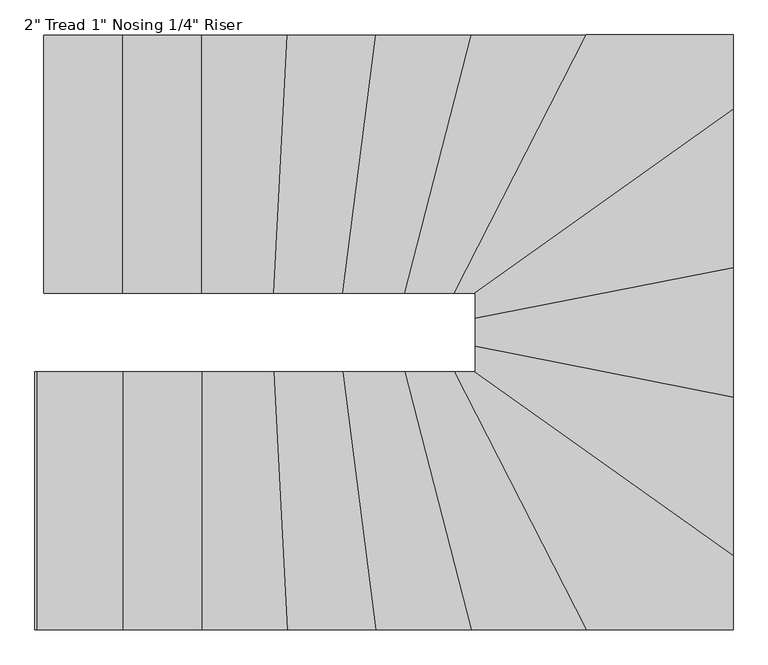
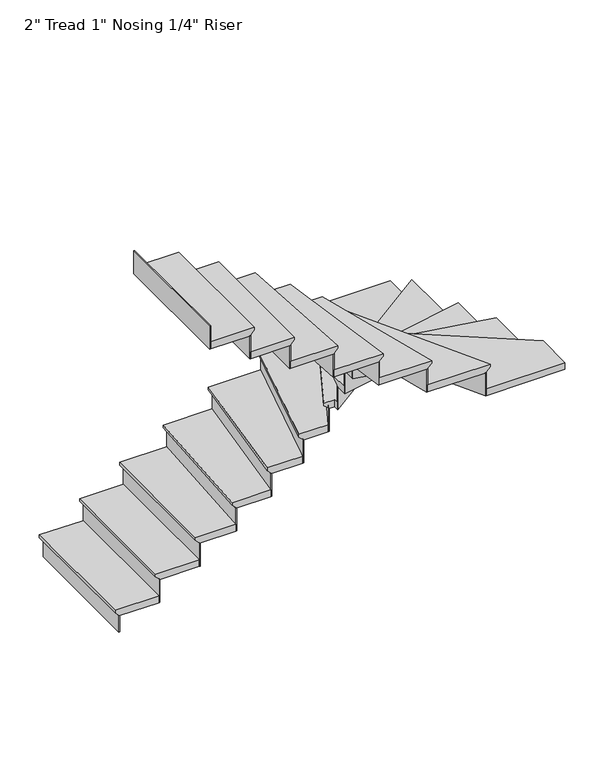
"""IFC4 building model written with IfcOpenShell, lengths in millimetres: stair flight geometry."""

from ifc_helpers import new_model, si_unit, origin, place, context, project, spatial, faceted_brep, source, transform, mapped, element, save


def stair_flight_813748e6(model_context):
    return source(origin(), model_context, "Body", "Brep", [
        faceted_brep([(-5314.5158104, 2778.8271763, 150.2833333), (-5314.5158104, 2778.8271763, 169.3333333), (-5314.5158104, 3693.2271763, 169.3333333), (-5314.5158104, 3693.2271763, 150.2833333), (-5289.1158104, 2778.8271763, 124.8833333), (-5289.1158104, 3693.2271763, 124.8833333), (-5009.7158104, 2778.8271763, 169.3333333), (-5009.7158104, 3693.2271763, 169.3333333), (-5289.1158104, 3693.2271763, 118.5333333), (-5009.7158104, 3693.2271763, 118.5333333), (-5009.7158104, 2778.8271763, 118.5333333), (-5289.1158104, 2778.8271763, 118.5333333)], [[[0, 1, 2, 3]], [[4, 0, 3, 5]], [[2, 1, 6, 7]], [[8, 9, 10, 11]], [[2, 7, 9, 8, 5, 3]], [[8, 11, 4, 5]], [[6, 1, 0, 4, 11, 10]], [[7, 6, 10, 9]]]),
        faceted_brep([(-5289.1158104, 2778.8271763, 118.5333333), (-5289.1158104, 2778.8271763, 0.0), (-5282.7658104, 2778.8271763, 0.0), (-5282.7658104, 2778.8271763, 118.5333333), (-5289.1158104, 3693.2271763, 118.5333333), (-5282.7658104, 3693.2271763, 118.5333333), (-5282.7658104, 3693.2271763, 0.0), (-5289.1158104, 3693.2271763, 0.0)], [[[0, 1, 2, 3]], [[4, 5, 6, 7]], [[1, 0, 4, 7]], [[2, 1, 7, 6]], [[3, 2, 6, 5]], [[0, 3, 5, 4]]]),
        faceted_brep([(-5009.7158104, 2778.8271763, 287.8666667), (-5009.7158104, 2778.8271763, 118.5333333), (-5003.3658104, 2778.8271763, 118.5333333), (-5003.3658104, 2778.8271763, 287.8666667), (-5009.7158104, 3693.2271763, 287.8666667), (-5003.3658104, 3693.2271763, 287.8666667), (-5003.3658104, 3693.2271763, 118.5333333), (-5009.7158104, 3693.2271763, 118.5333333)], [[[0, 1, 2, 3]], [[4, 5, 6, 7]], [[1, 0, 4, 7]], [[2, 1, 7, 6]], [[3, 2, 6, 5]], [[0, 3, 5, 4]]]),
        faceted_brep([(-5035.1158104, 3693.2271763, 338.6666667), (-5035.1158104, 2778.8271763, 338.6666667), (-4730.3158104, 2778.8271763, 338.6666667), (-4730.3158104, 3693.2271763, 338.6666667), (-5009.7158104, 3693.2271763, 287.8666667), (-4730.3158104, 3693.2271763, 287.8666667), (-4730.3158104, 2778.8271763, 287.8666667), (-5009.7158104, 2778.8271763, 287.8666667), (-5009.7158104, 3693.2271763, 294.2166667), (-5035.1158104, 3693.2271763, 319.6166667), (-5009.7158104, 2778.8271763, 294.2166667), (-5035.1158104, 2778.8271763, 319.6166667)], [[[0, 1, 2, 3]], [[4, 5, 6, 7]], [[0, 3, 5, 4, 8, 9]], [[4, 7, 10, 8]], [[2, 1, 11, 10, 7, 6]], [[3, 2, 6, 5]], [[11, 1, 0, 9]], [[10, 11, 9, 8]]]),
        faceted_brep([(-4730.3158104, 2778.8271763, 457.2), (-4730.3158104, 2778.8271763, 287.8666667), (-4723.9658104, 2778.8271763, 287.8666667), (-4723.9658104, 2778.8271763, 457.2), (-4730.3158104, 3693.2271763, 457.2), (-4723.9658104, 3693.2271763, 457.2), (-4723.9658104, 3693.2271763, 287.8666667), (-4730.3158104, 3693.2271763, 287.8666667)], [[[0, 1, 2, 3]], [[4, 5, 6, 7]], [[1, 0, 4, 7]], [[2, 1, 7, 6]], [[3, 2, 6, 5]], [[0, 3, 5, 4]]]),
        faceted_brep([(-4755.7158104, 3693.2271763, 508.0), (-4755.7158104, 2778.8271763, 508.0), (-4474.6486489, 2778.8271763, 508.0), (-4427.1143785, 3693.2271763, 508.0), (-4730.3158104, 3693.2271763, 457.2), (-4427.1143785, 3693.2271763, 457.2), (-4474.6486489, 2778.8271763, 457.2), (-4730.3158104, 2778.8271763, 457.2), (-4730.3158104, 3693.2271763, 463.55), (-4755.7158104, 3693.2271763, 488.95), (-4730.3158104, 2778.8271763, 463.55), (-4755.7158104, 2778.8271763, 488.95)], [[[0, 1, 2, 3]], [[4, 5, 6, 7]], [[0, 3, 5, 4, 8, 9]], [[4, 7, 10, 8]], [[2, 1, 11, 10, 7, 6]], [[3, 2, 6, 5]], [[11, 1, 0, 9]], [[10, 11, 9, 8]]]),
        faceted_brep([(-4474.6486489, 2778.8271763, 626.5333333), (-4474.6486489, 2778.8271763, 457.2), (-4468.2900747, 2778.8271763, 457.2), (-4468.2900747, 2778.8271763, 626.5333333), (-4427.1143785, 3693.2271763, 626.5333333), (-4420.7558043, 3693.2271763, 626.5333333), (-4420.7558043, 3693.2271763, 457.2), (-4427.1143785, 3693.2271763, 457.2)], [[[0, 1, 2, 3]], [[4, 5, 6, 7]], [[1, 0, 4, 7]], [[2, 1, 7, 6]], [[3, 2, 6, 5]], [[0, 3, 5, 4]]]),
        faceted_brep([(-4452.5486752, 3693.2271763, 677.3333333), (-4500.0829456, 2778.8271763, 677.3333333), (-4230.4819491, 2778.8271763, 677.3333333), (-4112.1258974, 3693.2271763, 677.3333333), (-4427.1143785, 3693.2271763, 626.5333333), (-4112.1258974, 3693.2271763, 626.5333333), (-4230.4819491, 2778.8271763, 626.5333333), (-4474.6486489, 2778.8271763, 626.5333333), (-4427.1143785, 3693.2271763, 632.8833333), (-4452.5486752, 3693.2271763, 658.2833333), (-4474.6486489, 2778.8271763, 632.8833333), (-4500.0829456, 2778.8271763, 658.2833333)], [[[0, 1, 2, 3]], [[4, 5, 6, 7]], [[0, 3, 5, 4, 8, 9]], [[4, 7, 10, 8]], [[2, 1, 11, 10, 7, 6]], [[3, 2, 6, 5]], [[11, 1, 0, 9]], [[10, 11, 9, 8]]]),
        faceted_brep([(-4230.4819491, 2778.8271763, 795.8666667), (-4230.4819491, 2778.8271763, 626.5333333), (-4224.0789773, 2778.8271763, 626.5333333), (-4224.0789773, 2778.8271763, 795.8666667), (-4112.1258974, 3693.2271763, 795.8666667), (-4105.7229256, 3693.2271763, 795.8666667), (-4105.7229256, 3693.2271763, 626.5333333), (-4112.1258974, 3693.2271763, 626.5333333)], [[[0, 1, 2, 3]], [[4, 5, 6, 7]], [[1, 0, 4, 7]], [[2, 1, 7, 6]], [[3, 2, 6, 5]], [[0, 3, 5, 4]]]),
        faceted_brep([(-4137.7377845, 3693.2271763, 846.6666667), (-4256.0938362, 2778.8271763, 846.6666667), (-4008.8547266, 2778.8271763, 846.6666667), (-3773.7242792, 3693.2271763, 846.6666667), (-4112.1258974, 3693.2271763, 795.8666667), (-3773.7242792, 3693.2271763, 795.8666667), (-4008.8547266, 2778.8271763, 795.8666667), (-4230.4819491, 2778.8271763, 795.8666667), (-4112.1258974, 3693.2271763, 802.2166667), (-4137.7377845, 3693.2271763, 827.6166667), (-4230.4819491, 2778.8271763, 802.2166667), (-4256.0938362, 2778.8271763, 827.6166667)], [[[0, 1, 2, 3]], [[4, 5, 6, 7]], [[0, 3, 5, 4, 8, 9]], [[4, 7, 10, 8]], [[2, 1, 11, 10, 7, 6]], [[3, 2, 6, 5]], [[11, 1, 0, 9]], [[10, 11, 9, 8]]]),
        faceted_brep([(-4008.8547266, 2778.8271763, 965.2), (-4008.8547266, 2778.8271763, 795.8666667), (-4002.2981497, 2778.8271763, 795.8666667), (-4002.2981497, 2778.8271763, 965.2), (-3773.7242792, 3693.2271763, 965.2), (-3767.1677023, 3693.2271763, 965.2), (-3767.1677023, 3693.2271763, 795.8666667), (-3773.7242792, 3693.2271763, 795.8666667)], [[[0, 1, 2, 3]], [[4, 5, 6, 7]], [[1, 0, 4, 7]], [[2, 1, 7, 6]], [[3, 2, 6, 5]], [[0, 3, 5, 4]]]),
        faceted_brep([(-3799.9505867, 3693.2271763, 1016.0), (-4035.0810341, 2778.8271763, 1016.0), (-3832.5080905, 2778.8271763, 1016.0), (-3363.6834692, 3693.2271763, 1016.0), (-3773.7242792, 3693.2271763, 965.2), (-3363.6834692, 3693.2271763, 965.2), (-3832.5080905, 2778.8271763, 965.2), (-4008.8547266, 2778.8271763, 965.2), (-3773.7242792, 3693.2271763, 971.55), (-3799.9505867, 3693.2271763, 996.95), (-4008.8547266, 2778.8271763, 971.55), (-4035.0810341, 2778.8271763, 996.95)], [[[0, 1, 2, 3]], [[4, 5, 6, 7]], [[0, 3, 5, 4, 8, 9]], [[4, 7, 10, 8]], [[2, 1, 11, 10, 7, 6]], [[3, 2, 6, 5]], [[11, 1, 0, 9]], [[10, 11, 9, 8]]]),
        faceted_brep([(-3832.5080905, 2778.8271763, 1134.5333333), (-3832.5080905, 2778.8271763, 965.2), (-3825.3721074, 2778.8271763, 965.2), (-3825.3721074, 2778.8271763, 1134.5333333), (-3363.6834692, 3693.2271763, 1134.5333333), (-3356.5474861, 3693.2271763, 1134.5333333), (-3356.5474861, 3693.2271763, 965.2), (-3363.6834692, 3693.2271763, 965.2)], [[[0, 1, 2, 3]], [[4, 5, 6, 7]], [[1, 0, 4, 7]], [[2, 1, 7, 6]], [[3, 2, 6, 5]], [[0, 3, 5, 4]]]),
        faceted_brep([(-2872.3841185, 3399.5460426, 1185.3333333), (-2872.3841185, 3693.2271763, 1185.3333333), (-3392.2274017, 3693.2271763, 1185.3333333), (-3861.0520231, 2778.8271763, 1185.3333333), (-3786.7841185, 2778.8271763, 1185.3333333), (-3786.7841185, 2749.2720934, 1185.3333333), (-2872.3841185, 3693.2271763, 1134.5333333), (-2872.3841185, 3399.5460426, 1134.5333333), (-3786.7841185, 2749.2720934, 1134.5333333), (-3786.7841185, 2778.8271763, 1134.5333333), (-3832.5080905, 2778.8271763, 1134.5333333), (-3363.6834692, 3693.2271763, 1134.5333333), (-3363.6834692, 3693.2271763, 1140.8833333), (-3392.2274017, 3693.2271763, 1166.2833333), (-3832.5080905, 2778.8271763, 1140.8833333), (-3861.0520231, 2778.8271763, 1166.2833333)], [[[0, 1, 2, 3, 4, 5]], [[6, 7, 8, 9, 10, 11]], [[1, 0, 7, 6]], [[2, 1, 6, 11, 12, 13]], [[11, 10, 14, 12]], [[4, 3, 15, 14, 10, 9]], [[5, 4, 9, 8]], [[0, 5, 8, 7]], [[15, 3, 2, 13]], [[14, 15, 13, 12]]]),
        faceted_brep([(-3786.7841185, 2749.2720934, 1303.8666667), (-3786.7841185, 2749.2720934, 1134.5333333), (-3786.7841185, 2741.4801186, 1134.5333333), (-3786.7841185, 2741.4801186, 1303.8666667), (-2872.3841185, 3399.5460426, 1303.8666667), (-2872.3841185, 3391.7540678, 1303.8666667), (-2872.3841185, 3391.7540678, 1134.5333333), (-2872.3841185, 3399.5460426, 1134.5333333)], [[[0, 1, 2, 3]], [[4, 5, 6, 7]], [[1, 0, 4, 7]], [[2, 1, 7, 6]], [[3, 2, 6, 5]], [[0, 3, 5, 4]]]),
        faceted_brep([(-2872.3841185, 3430.7139417, 1354.6666667), (-3786.7841185, 2780.4399926, 1354.6666667), (-3786.7841185, 2662.8180064, 1354.6666667), (-2872.3841185, 2843.0588627, 1354.6666667), (-2872.3841185, 3399.5460426, 1303.8666667), (-2872.3841185, 2843.0588627, 1303.8666667), (-3786.7841185, 2662.8180064, 1303.8666667), (-3786.7841185, 2749.2720934, 1303.8666667), (-2872.3841185, 3399.5460426, 1310.2166667), (-2872.3841185, 3430.7139417, 1335.6166667), (-3786.7841185, 2749.2720934, 1310.2166667), (-3786.7841185, 2780.4399926, 1335.6166667)], [[[0, 1, 2, 3]], [[4, 5, 6, 7]], [[0, 3, 5, 4, 8, 9]], [[4, 7, 10, 8]], [[2, 1, 11, 10, 7, 6]], [[3, 2, 6, 5]], [[11, 1, 0, 9]], [[10, 11, 9, 8]]]),
        faceted_brep([(-3786.7841185, 2662.8180064, 1473.2), (-3786.7841185, 2662.8180064, 1303.8666667), (-3786.7841185, 2656.3458209, 1303.8666667), (-3786.7841185, 2656.3458209, 1473.2), (-2872.3841185, 2843.0588627, 1473.2), (-2872.3841185, 2836.5866772, 1473.2), (-2872.3841185, 2836.5866772, 1303.8666667), (-2872.3841185, 2843.0588627, 1303.8666667)], [[[0, 1, 2, 3]], [[4, 5, 6, 7]], [[1, 0, 4, 7]], [[2, 1, 7, 6]], [[3, 2, 6, 5]], [[0, 3, 5, 4]]]),
        faceted_brep([(-2872.3841185, 2868.9476044, 1524.0), (-3786.7841185, 2688.7067481, 1524.0), (-3786.7841185, 2563.6588627, 1524.0), (-2872.3841185, 2383.4180064, 1524.0), (-2872.3841185, 2843.0588627, 1473.2), (-2872.3841185, 2383.4180064, 1473.2), (-3786.7841185, 2563.6588627, 1473.2), (-3786.7841185, 2662.8180064, 1473.2), (-2872.3841185, 2843.0588627, 1479.55), (-2872.3841185, 2868.9476044, 1504.95), (-3786.7841185, 2662.8180064, 1479.55), (-3786.7841185, 2688.7067481, 1504.95)], [[[0, 1, 2, 3]], [[4, 5, 6, 7]], [[0, 3, 5, 4, 8, 9]], [[4, 7, 10, 8]], [[2, 1, 11, 10, 7, 6]], [[3, 2, 6, 5]], [[11, 1, 0, 9]], [[10, 11, 9, 8]]]),
        faceted_brep([(-3786.7841185, 2563.6588627, 1642.5333333), (-3786.7841185, 2563.6588627, 1473.2), (-3786.7841185, 2557.1866772, 1473.2), (-3786.7841185, 2557.1866772, 1642.5333333), (-2872.3841185, 2383.4180064, 1642.5333333), (-2872.3841185, 2376.9458209, 1642.5333333), (-2872.3841185, 2376.9458209, 1473.2), (-2872.3841185, 2383.4180064, 1473.2)], [[[0, 1, 2, 3]], [[4, 5, 6, 7]], [[1, 0, 4, 7]], [[2, 1, 7, 6]], [[3, 2, 6, 5]], [[0, 3, 5, 4]]]),
        faceted_brep([(-2872.3841185, 2409.3067481, 1693.3333333), (-3786.7841185, 2589.5476044, 1693.3333333), (-3786.7841185, 2499.4271763, 1693.3333333), (-3832.879593, 2499.4271763, 1693.3333333), (-2872.3841185, 1816.3725116, 1693.3333333), (-2872.3841185, 2383.4180064, 1642.5333333), (-2872.3841185, 1816.3725116, 1642.5333333), (-3832.879593, 2499.4271763, 1642.5333333), (-3786.7841185, 2499.4271763, 1642.5333333), (-3786.7841185, 2563.6588627, 1642.5333333), (-2872.3841185, 2383.4180064, 1648.8833333), (-2872.3841185, 2409.3067481, 1674.2833333), (-3786.7841185, 2563.6588627, 1648.8833333), (-3786.7841185, 2589.5476044, 1674.2833333)], [[[0, 1, 2, 3, 4]], [[5, 6, 7, 8, 9]], [[0, 4, 6, 5, 10, 11]], [[5, 9, 12, 10]], [[2, 1, 13, 12, 9, 8]], [[3, 2, 8, 7]], [[4, 3, 7, 6]], [[13, 1, 0, 11]], [[12, 13, 11, 10]]]),
        faceted_brep([(-3832.879593, 2499.4271763, 1811.8666667), (-3832.879593, 2499.4271763, 1642.5333333), (-3843.8364855, 2499.4271763, 1642.5333333), (-3843.8364855, 2499.4271763, 1811.8666667), (-2872.3841185, 1816.3725116, 1811.8666667), (-2872.3841185, 1808.5805368, 1811.8666667), (-2872.3841185, 1808.5805368, 1642.5333333), (-2872.3841185, 1816.3725116, 1642.5333333)], [[[0, 1, 2, 3]], [[4, 5, 6, 7]], [[1, 0, 4, 7]], [[2, 1, 7, 6]], [[3, 2, 6, 5]], [[0, 3, 5, 4]]]),
        faceted_brep([(-3420.7713343, 1585.0271763, 1862.6666667), (-2872.3841185, 1585.0271763, 1862.6666667), (-2872.3841185, 1847.5404108, 1862.6666667), (-3789.0520231, 2499.4271763, 1862.6666667), (-3889.5959556, 2499.4271763, 1862.6666667), (-2872.3841185, 1585.0271763, 1811.8666667), (-3420.7713343, 1585.0271763, 1811.8666667), (-3889.5959556, 2499.4271763, 1811.8666667), (-3832.879593, 2499.4271763, 1811.8666667), (-2872.3841185, 1816.3725116, 1811.8666667), (-2872.3841185, 1816.3725116, 1818.2166667), (-2872.3841185, 1847.5404108, 1843.6166667), (-3832.879593, 2499.4271763, 1818.2166667), (-3789.0520231, 2499.4271763, 1843.6166667)], [[[0, 1, 2, 3, 4]], [[5, 6, 7, 8, 9]], [[1, 0, 6, 5]], [[2, 1, 5, 9, 10, 11]], [[9, 8, 12, 10]], [[4, 3, 13, 12, 8, 7]], [[0, 4, 7, 6]], [[13, 3, 2, 11]], [[12, 13, 11, 10]]]),
        faceted_brep([(-3889.5959556, 2499.4271763, 1981.2), (-3889.5959556, 2499.4271763, 1811.8666667), (-3896.7319387, 2499.4271763, 1811.8666667), (-3896.7319387, 2499.4271763, 1981.2), (-3420.7713343, 1585.0271763, 1981.2), (-3427.9073174, 1585.0271763, 1981.2), (-3427.9073174, 1585.0271763, 1811.8666667), (-3420.7713343, 1585.0271763, 1811.8666667)], [[[0, 1, 2, 3]], [[4, 5, 6, 7]], [[1, 0, 4, 7]], [[2, 1, 7, 6]], [[3, 2, 6, 5]], [[0, 3, 5, 4]]]),
        faceted_brep([(-3392.2274017, 1585.0271763, 2032.0), (-3861.0520231, 2499.4271763, 2032.0), (-4061.3073415, 2499.4271763, 2032.0), (-3826.1768941, 1585.0271763, 2032.0), (-3420.7713343, 1585.0271763, 1981.2), (-3826.1768941, 1585.0271763, 1981.2), (-4061.3073415, 2499.4271763, 1981.2), (-3889.5959556, 2499.4271763, 1981.2), (-3420.7713343, 1585.0271763, 1987.55), (-3392.2274017, 1585.0271763, 2012.95), (-3889.5959556, 2499.4271763, 1987.55), (-3861.0520231, 2499.4271763, 2012.95)], [[[0, 1, 2, 3]], [[4, 5, 6, 7]], [[0, 3, 5, 4, 8, 9]], [[4, 7, 10, 8]], [[2, 1, 11, 10, 7, 6]], [[3, 2, 6, 5]], [[11, 1, 0, 9]], [[10, 11, 9, 8]]]),
        faceted_brep([(-4061.3073415, 2499.4271763, 2150.5333333), (-4061.3073415, 2499.4271763, 1981.2), (-4067.8639184, 2499.4271763, 1981.2), (-4067.8639184, 2499.4271763, 2150.5333333), (-3826.1768941, 1585.0271763, 2150.5333333), (-3832.733471, 1585.0271763, 2150.5333333), (-3832.733471, 1585.0271763, 1981.2), (-3826.1768941, 1585.0271763, 1981.2)], [[[0, 1, 2, 3]], [[4, 5, 6, 7]], [[1, 0, 4, 7]], [[2, 1, 7, 6]], [[3, 2, 6, 5]], [[0, 3, 5, 4]]]),
        faceted_brep([(-3799.9505867, 1585.0271763, 2201.3333333), (-4035.0810341, 2499.4271763, 2201.3333333), (-4281.7057233, 2499.4271763, 2201.3333333), (-4163.3496716, 1585.0271763, 2201.3333333), (-3826.1768941, 1585.0271763, 2150.5333333), (-4163.3496716, 1585.0271763, 2150.5333333), (-4281.7057233, 2499.4271763, 2150.5333333), (-4061.3073415, 2499.4271763, 2150.5333333), (-3826.1768941, 1585.0271763, 2156.8833333), (-3799.9505867, 1585.0271763, 2182.2833333), (-4061.3073415, 2499.4271763, 2156.8833333), (-4035.0810341, 2499.4271763, 2182.2833333)], [[[0, 1, 2, 3]], [[4, 5, 6, 7]], [[0, 3, 5, 4, 8, 9]], [[4, 7, 10, 8]], [[2, 1, 11, 10, 7, 6]], [[3, 2, 6, 5]], [[11, 1, 0, 9]], [[10, 11, 9, 8]]]),
        faceted_brep([(-4281.7057233, 2499.4271763, 2319.8666667), (-4281.7057233, 2499.4271763, 2150.5333333), (-4288.1086951, 2499.4271763, 2150.5333333), (-4288.1086951, 2499.4271763, 2319.8666667), (-4163.3496716, 1585.0271763, 2319.8666667), (-4169.7526434, 1585.0271763, 2319.8666667), (-4169.7526434, 1585.0271763, 2150.5333333), (-4163.3496716, 1585.0271763, 2150.5333333)], [[[0, 1, 2, 3]], [[4, 5, 6, 7]], [[1, 0, 4, 7]], [[2, 1, 7, 6]], [[3, 2, 6, 5]], [[0, 3, 5, 4]]]),
        faceted_brep([(-4137.7377845, 1585.0271763, 2370.6666667), (-4256.0938362, 2499.4271763, 2370.6666667), (-4525.5172422, 2499.4271763, 2370.6666667), (-4477.9829718, 1585.0271763, 2370.6666667), (-4163.3496716, 1585.0271763, 2319.8666667), (-4477.9829718, 1585.0271763, 2319.8666667), (-4525.5172422, 2499.4271763, 2319.8666667), (-4281.7057233, 2499.4271763, 2319.8666667), (-4163.3496716, 1585.0271763, 2326.2166667), (-4137.7377845, 1585.0271763, 2351.6166667), (-4281.7057233, 2499.4271763, 2326.2166667), (-4256.0938362, 2499.4271763, 2351.6166667)], [[[0, 1, 2, 3]], [[4, 5, 6, 7]], [[0, 3, 5, 4, 8, 9]], [[4, 7, 10, 8]], [[2, 1, 11, 10, 7, 6]], [[3, 2, 6, 5]], [[11, 1, 0, 9]], [[10, 11, 9, 8]]]),
        faceted_brep([(-4525.5172422, 2499.4271763, 2489.2), (-4525.5172422, 2499.4271763, 2319.8666667), (-4531.8758164, 2499.4271763, 2319.8666667), (-4531.8758164, 2499.4271763, 2489.2), (-4477.9829718, 1585.0271763, 2489.2), (-4484.341546, 1585.0271763, 2489.2), (-4484.341546, 1585.0271763, 2319.8666667), (-4477.9829718, 1585.0271763, 2319.8666667)], [[[0, 1, 2, 3]], [[4, 5, 6, 7]], [[1, 0, 4, 7]], [[2, 1, 7, 6]], [[3, 2, 6, 5]], [[0, 3, 5, 4]]]),
        faceted_brep([(-4452.5486752, 1585.0271763, 2540.0), (-4500.0829456, 2499.4271763, 2540.0), (-4781.1158104, 2499.4271763, 2540.0), (-4781.1158104, 1585.0271763, 2540.0), (-4477.9829718, 1585.0271763, 2489.2), (-4781.1158104, 1585.0271763, 2489.2), (-4781.1158104, 2499.4271763, 2489.2), (-4525.5172422, 2499.4271763, 2489.2), (-4477.9829718, 1585.0271763, 2495.55), (-4452.5486752, 1585.0271763, 2520.95), (-4525.5172422, 2499.4271763, 2495.55), (-4500.0829456, 2499.4271763, 2520.95)], [[[0, 1, 2, 3]], [[4, 5, 6, 7]], [[0, 3, 5, 4, 8, 9]], [[4, 7, 10, 8]], [[2, 1, 11, 10, 7, 6]], [[3, 2, 6, 5]], [[11, 1, 0, 9]], [[10, 11, 9, 8]]]),
        faceted_brep([(-4781.1158104, 2499.4271763, 2658.5333333), (-4781.1158104, 2499.4271763, 2489.2), (-4787.4658104, 2499.4271763, 2489.2), (-4787.4658104, 2499.4271763, 2658.5333333), (-4781.1158104, 1585.0271763, 2658.5333333), (-4787.4658104, 1585.0271763, 2658.5333333), (-4787.4658104, 1585.0271763, 2489.2), (-4781.1158104, 1585.0271763, 2489.2)], [[[0, 1, 2, 3]], [[4, 5, 6, 7]], [[1, 0, 4, 7]], [[2, 1, 7, 6]], [[3, 2, 6, 5]], [[0, 3, 5, 4]]]),
        faceted_brep([(-4755.7158104, 1585.0271763, 2709.3333333), (-4755.7158104, 2499.4271763, 2709.3333333), (-5060.5158104, 2499.4271763, 2709.3333333), (-5060.5158104, 1585.0271763, 2709.3333333), (-4781.1158104, 1585.0271763, 2658.5333333), (-5060.5158104, 1585.0271763, 2658.5333333), (-5060.5158104, 2499.4271763, 2658.5333333), (-4781.1158104, 2499.4271763, 2658.5333333), (-4781.1158104, 1585.0271763, 2664.8833333), (-4755.7158104, 1585.0271763, 2690.2833333), (-4781.1158104, 2499.4271763, 2664.8833333), (-4755.7158104, 2499.4271763, 2690.2833333)], [[[0, 1, 2, 3]], [[4, 5, 6, 7]], [[0, 3, 5, 4, 8, 9]], [[4, 7, 10, 8]], [[2, 1, 11, 10, 7, 6]], [[3, 2, 6, 5]], [[11, 1, 0, 9]], [[10, 11, 9, 8]]]),
        faceted_brep([(-5060.5158104, 2499.4271763, 2827.8666667), (-5060.5158104, 2499.4271763, 2658.5333333), (-5066.8658104, 2499.4271763, 2658.5333333), (-5066.8658104, 2499.4271763, 2827.8666667), (-5060.5158104, 1585.0271763, 2827.8666667), (-5066.8658104, 1585.0271763, 2827.8666667), (-5066.8658104, 1585.0271763, 2658.5333333), (-5060.5158104, 1585.0271763, 2658.5333333)], [[[0, 1, 2, 3]], [[4, 5, 6, 7]], [[1, 0, 4, 7]], [[2, 1, 7, 6]], [[3, 2, 6, 5]], [[0, 3, 5, 4]]]),
        faceted_brep([(-5339.9158104, 2499.4271763, 2997.2), (-5339.9158104, 2499.4271763, 2827.8666667), (-5346.2658104, 2499.4271763, 2827.8666667), (-5346.2658104, 2499.4271763, 2997.2), (-5339.9158104, 1585.0271763, 2997.2), (-5346.2658104, 1585.0271763, 2997.2), (-5346.2658104, 1585.0271763, 2827.8666667), (-5339.9158104, 1585.0271763, 2827.8666667)], [[[0, 1, 2, 3]], [[4, 5, 6, 7]], [[1, 0, 4, 7]], [[2, 1, 7, 6]], [[3, 2, 6, 5]], [[0, 3, 5, 4]]]),
        faceted_brep([(-5035.1158104, 1585.0271763, 2878.6666667), (-5035.1158104, 2499.4271763, 2878.6666667), (-5339.9158104, 2499.4271763, 2878.6666667), (-5339.9158104, 1585.0271763, 2878.6666667), (-5060.5158104, 1585.0271763, 2827.8666667), (-5339.9158104, 1585.0271763, 2827.8666667), (-5339.9158104, 2499.4271763, 2827.8666667), (-5060.5158104, 2499.4271763, 2827.8666667), (-5060.5158104, 1585.0271763, 2834.2166667), (-5035.1158104, 1585.0271763, 2859.6166667), (-5060.5158104, 2499.4271763, 2834.2166667), (-5035.1158104, 2499.4271763, 2859.6166667)], [[[0, 1, 2, 3]], [[4, 5, 6, 7]], [[0, 3, 5, 4, 8, 9]], [[4, 7, 10, 8]], [[2, 1, 11, 10, 7, 6]], [[3, 2, 6, 5]], [[11, 1, 0, 9]], [[10, 11, 9, 8]]]),
    ])


if __name__ == "__main__":
    model = new_model("IFC4")
    model_context = context("Model", 3, world=origin())
    ifc_project = project(units=[si_unit("LENGTHUNIT", "METRE", prefix="MILLI")], contexts=[model_context])
    site = spatial("IfcSite", under=ifc_project)
    building = spatial("IfcBuilding", under=site)
    placement = place(None, origin())
    stair_flight_shape = stair_flight_813748e6(model_context)
    element("IfcStairFlight", 1, ObjectType="2\" Tread 1\" Nosing 1/4\" Riser", at=placement, inside=building, context=model_context, shape_type="MappedRepresentation", body=[
        mapped(stair_flight_shape, transform((0.0, 0.0, 0.0), x_axis=(1.0, 0.0, 0.0), y_axis=(0.0, 1.0, 0.0), z_axis=(0.0, 0.0, 1.0))),
    ])
    save(model, "model.ifc")
